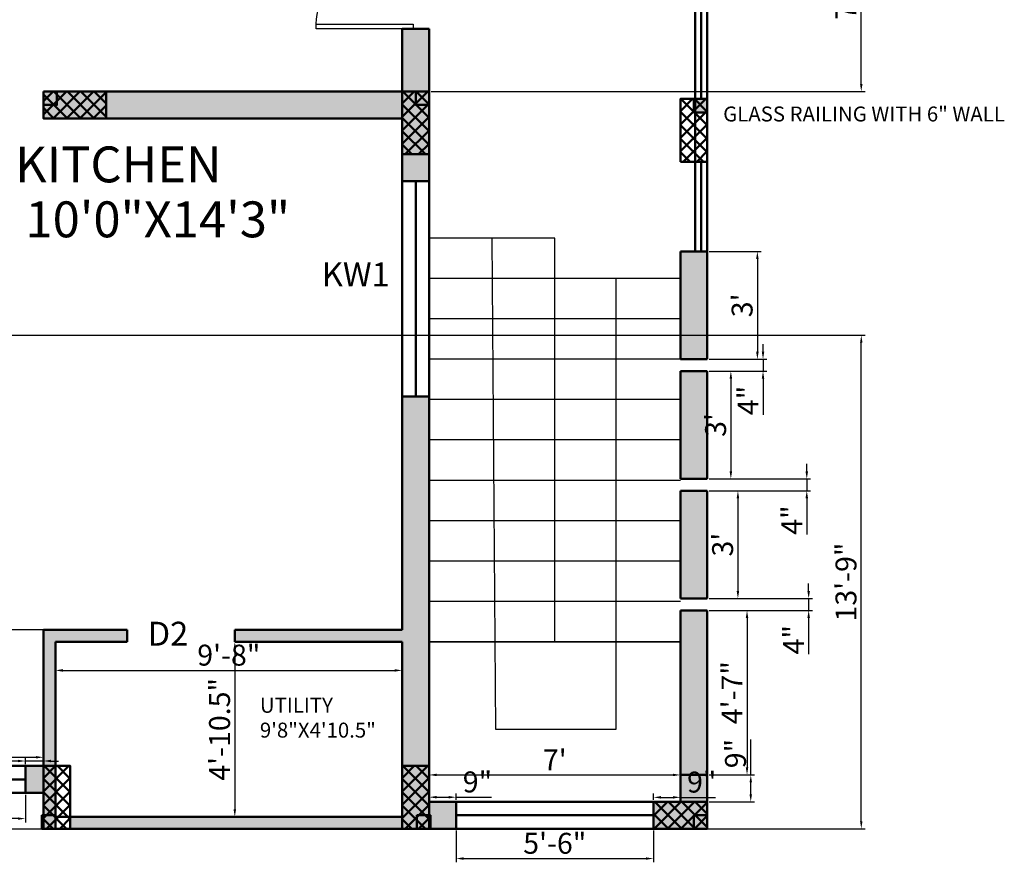
# Model space of a CAD drawing. Units: inches. Extents: x 1749 to 3550, y 1117 to 2383.
# Tile 4 of 15: x 2277 to 2606, y 1199 to 1481. Entities that reach past the tile are written whole.
import ezdxf

# ---------------------------------------------------------------- set-up
doc = ezdxf.new("R2010")
doc.units = ezdxf.units.IN
for name, color, linetype, lineweight in [('A-ANNO-DIMS', 2, 'Continuous', 18), ('A-ANNO-TEXT', 3, 'Continuous', 18), ('A-AREA-IDEN', 7, 'Continuous', 18), ('A-COLS', 10, 'Continuous', 50), ('A-DOOR', 30, 'Continuous', 25), ('A-FLOR-STRS', 53, 'Continuous', 25), ('A-WALL', 7, 'Continuous', 50), ('A-WALL-PATT', 8, 'Continuous', 13)]:
    doc.layers.add(name, color=color, linetype=linetype, lineweight=lineweight)
doc.styles.get("Standard").update_dxf_attribs({"font": 'arial.ttf'})
doc.dimstyles.new('ISO-25', dxfattribs={"dimtxt": 7, "dimasz": 2.5, "dimexe": 1.25, "dimexo": 0.625, "dimtad": 1, "dimdec": 1, "dimlunit": 3, "dimtxsty": 'Standard', "dimcen": 2.5, "dimadec": 0, "dimazin": 0, "dimtfac": 1, "dimtdec": 1, "dimtmove": 0, "dimatfit": 3, "dimfxl": 1, "dimarcsym": 0})

# ---------------------------------------------------------------- blocks, each defined once
blk = doc.blocks.new('*U14')
for p, q in [((0, 0), (0, 6)), ((36, 0), (36, 6))]:
    blk.add_line(p, q)
blk.add_lwpolyline([(0, 0), (0, -36), (1.75, -36), (1.75, 0)], close=True)
blk.add_arc((0, 0), 36, 270, 0)
blk = doc.blocks.new('*D27')
at = {"layer": 'A-ANNO-DIMS', "color": 0, "lineweight": -2, "ltscale": 0.5, "transparency": 16777216}
for p, q in [((2349.73, 1272.74), (2350.35, 1272.74)), ((2349.1, 1270.24), (2349.1, 1216.74)), ((2349.73, 1214.24), (2350.35, 1214.24))]:
    blk.add_line(p, q, dxfattribs=at)
at = {"layer": 'A-ANNO-DIMS', "color": 0, "ltscale": 0.5, "transparency": 16777216}
for points in [[(2348.69, 1270.24), (2349.52, 1270.24), (2349.1, 1272.74)], [(2348.69, 1216.74), (2349.52, 1216.74), (2349.1, 1214.24)]]:
    blk.add_solid(points, dxfattribs=at)
at = {"layer": 'Defpoints', "color": 0, "ltscale": 0.5, "transparency": 16777216}
for p in [(2349.1, 1272.74), (2349.1, 1214.24), (2349.1, 1214.24)]:
    blk.add_point(p, dxfattribs=at)
at = {"layer": 'A-ANNO-DIMS', "color": 0, "ltscale": 0.5, "transparency": 16777216, "insert": (2344.91, 1243.49), "char_height": 7, "attachment_point": 5, "rotation": 90}
blk.add_mtext('4\'-10.5"', dxfattribs=at)
blk = doc.blocks.new('*D28')
at = {"layer": 'A-ANNO-DIMS', "color": 0, "lineweight": -2, "ltscale": 0.5, "transparency": 16777216}
for p, q in [((2289.1, 1272.12), (2289.1, 1261.94)), ((2405.1, 1272.12), (2405.1, 1261.94)), ((2291.6, 1263.19), (2402.6, 1263.19))]:
    blk.add_line(p, q, dxfattribs=at)
at = {"layer": 'A-ANNO-DIMS', "color": 0, "ltscale": 0.5, "transparency": 16777216}
for points in [[(2291.6, 1263.61), (2291.6, 1262.77), (2289.1, 1263.19)], [(2402.6, 1263.61), (2402.6, 1262.77), (2405.1, 1263.19)]]:
    blk.add_solid(points, dxfattribs=at)
at = {"layer": 'Defpoints', "color": 0, "ltscale": 0.5, "transparency": 16777216}
for p in [(2289.1, 1272.74), (2405.1, 1272.74), (2405.1, 1263.19)]:
    blk.add_point(p, dxfattribs=at)
at = {"layer": 'A-ANNO-DIMS', "color": 0, "ltscale": 0.5, "transparency": 16777216, "insert": (2347.1, 1267.39), "char_height": 7, "attachment_point": 5}
blk.add_mtext('9\'-8"', dxfattribs=at)
blk = doc.blocks.new('*D29')
at = {"layer": 'A-ANNO-DIMS', "color": 0, "lineweight": -2, "ltscale": 0.5, "transparency": 16777216}
for p, q in [((2414.1, 1219.87), (2414.1, 1229.49)), ((2416.6, 1228.24), (2495.6, 1228.24)), ((2498.1, 1219.87), (2498.1, 1229.49))]:
    blk.add_line(p, q, dxfattribs=at)
at = {"layer": 'A-ANNO-DIMS', "color": 0, "ltscale": 0.5, "transparency": 16777216}
for points in [[(2416.6, 1228.66), (2416.6, 1227.83), (2414.1, 1228.24)], [(2495.6, 1228.66), (2495.6, 1227.83), (2498.1, 1228.24)]]:
    blk.add_solid(points, dxfattribs=at)
at = {"layer": 'Defpoints', "color": 0, "ltscale": 0.5, "transparency": 16777216}
for p in [(2498.1, 1228.24), (2414.1, 1219.24), (2498.1, 1219.24)]:
    blk.add_point(p, dxfattribs=at)
at = {"layer": 'A-ANNO-DIMS', "color": 0, "ltscale": 0.5, "transparency": 16777216, "insert": (2456.1, 1232.37), "char_height": 7, "attachment_point": 5}
blk.add_mtext("7'", dxfattribs=at)
blk = doc.blocks.new('*D43')
at = {"layer": 'A-ANNO-DIMS', "color": 0, "lineweight": -2, "ltscale": 0.5, "transparency": 16777216}
for p, q in [((2507.73, 1403.24), (2525.11, 1403.24)), ((2523.86, 1400.74), (2523.86, 1369.74)), ((2507.73, 1367.24), (2525.11, 1367.24))]:
    blk.add_line(p, q, dxfattribs=at)
at = {"layer": 'A-ANNO-DIMS', "color": 0, "ltscale": 0.5, "transparency": 16777216}
for points in [[(2523.44, 1400.74), (2524.28, 1400.74), (2523.86, 1403.24)], [(2523.44, 1369.74), (2524.28, 1369.74), (2523.86, 1367.24)]]:
    blk.add_solid(points, dxfattribs=at)
at = {"layer": 'Defpoints', "color": 0, "ltscale": 0.5, "transparency": 16777216}
for p in [(2507.1, 1403.24), (2507.1, 1367.24), (2523.86, 1367.24)]:
    blk.add_point(p, dxfattribs=at)
at = {"layer": 'A-ANNO-DIMS', "color": 0, "ltscale": 0.5, "transparency": 16777216, "insert": (2519.66, 1385.24), "char_height": 7, "attachment_point": 5, "rotation": 90}
blk.add_mtext("3'", dxfattribs=at)
blk = doc.blocks.new('*D44')
at = {"layer": 'A-ANNO-DIMS', "color": 0, "lineweight": -2, "ltscale": 0.5, "transparency": 16777216}
for p, q in [((2525.75, 1369.74), (2525.75, 1372.24)), ((2507.73, 1367.24), (2527, 1367.24)), ((2525.75, 1367.24), (2525.75, 1363.24)), ((2507.73, 1363.24), (2527, 1363.24)), ((2525.75, 1360.74), (2525.75, 1348.67))]:
    blk.add_line(p, q, dxfattribs=at)
at = {"layer": 'A-ANNO-DIMS', "color": 0, "ltscale": 0.5, "transparency": 16777216}
for points in [[(2525.33, 1369.74), (2526.16, 1369.74), (2525.75, 1367.24)], [(2525.33, 1360.74), (2526.16, 1360.74), (2525.75, 1363.24)]]:
    blk.add_solid(points, dxfattribs=at)
at = {"layer": 'Defpoints', "color": 0, "ltscale": 0.5, "transparency": 16777216}
for p in [(2507.1, 1367.24), (2507.1, 1363.24), (2525.75, 1363.24)]:
    blk.add_point(p, dxfattribs=at)
at = {"layer": 'A-ANNO-DIMS', "color": 0, "ltscale": 0.5, "transparency": 16777216, "insert": (2521.62, 1353.45), "char_height": 7, "attachment_point": 5, "rotation": 90}
blk.add_mtext('4"', dxfattribs=at)
blk = doc.blocks.new('*D45')
at = {"layer": 'A-ANNO-DIMS', "color": 0, "lineweight": -2, "ltscale": 0.5, "transparency": 16777216}
for p, q in [((2507.73, 1363.24), (2516.25, 1363.24)), ((2515, 1360.74), (2515, 1329.74)), ((2507.73, 1327.24), (2516.25, 1327.24))]:
    blk.add_line(p, q, dxfattribs=at)
at = {"layer": 'A-ANNO-DIMS', "color": 0, "ltscale": 0.5, "transparency": 16777216}
for points in [[(2514.58, 1360.74), (2515.41, 1360.74), (2515, 1363.24)], [(2514.58, 1329.74), (2515.41, 1329.74), (2515, 1327.24)]]:
    blk.add_solid(points, dxfattribs=at)
at = {"layer": 'Defpoints', "color": 0, "ltscale": 0.5, "transparency": 16777216}
for p in [(2507.1, 1363.24), (2507.1, 1327.24), (2515, 1327.24)]:
    blk.add_point(p, dxfattribs=at)
at = {"layer": 'A-ANNO-DIMS', "color": 0, "ltscale": 0.5, "transparency": 16777216, "insert": (2510.79, 1345.24), "char_height": 7, "attachment_point": 5, "rotation": 90}
blk.add_mtext("3'", dxfattribs=at)
blk = doc.blocks.new('*D46')
at = {"layer": 'A-ANNO-DIMS', "color": 0, "lineweight": -2, "ltscale": 0.5, "transparency": 16777216}
for p, q in [((2540.38, 1329.74), (2540.38, 1332.24)), ((2507.73, 1327.24), (2541.63, 1327.24)), ((2540.38, 1327.24), (2540.38, 1323.24)), ((2507.73, 1323.24), (2541.63, 1323.24)), ((2540.38, 1320.74), (2540.38, 1308.67))]:
    blk.add_line(p, q, dxfattribs=at)
at = {"layer": 'A-ANNO-DIMS', "color": 0, "ltscale": 0.5, "transparency": 16777216}
for points in [[(2539.96, 1329.74), (2540.8, 1329.74), (2540.38, 1327.24)], [(2539.96, 1320.74), (2540.8, 1320.74), (2540.38, 1323.24)]]:
    blk.add_solid(points, dxfattribs=at)
at = {"layer": 'Defpoints', "color": 0, "ltscale": 0.5, "transparency": 16777216}
for p in [(2507.1, 1327.24), (2507.1, 1323.24), (2540.38, 1323.24)]:
    blk.add_point(p, dxfattribs=at)
at = {"layer": 'A-ANNO-DIMS', "color": 0, "ltscale": 0.5, "transparency": 16777216, "insert": (2536.25, 1313.45), "char_height": 7, "attachment_point": 5, "rotation": 90}
blk.add_mtext('4"', dxfattribs=at)
blk = doc.blocks.new('*D47')
at = {"layer": 'A-ANNO-DIMS', "color": 0, "lineweight": -2, "ltscale": 0.5, "transparency": 16777216}
for p, q in [((2507.73, 1323.24), (2518.6, 1323.24)), ((2517.35, 1320.74), (2517.35, 1289.74)), ((2507.73, 1287.24), (2518.6, 1287.24))]:
    blk.add_line(p, q, dxfattribs=at)
at = {"layer": 'A-ANNO-DIMS', "color": 0, "ltscale": 0.5, "transparency": 16777216}
for points in [[(2516.93, 1320.74), (2517.76, 1320.74), (2517.35, 1323.24)], [(2516.93, 1289.74), (2517.76, 1289.74), (2517.35, 1287.24)]]:
    blk.add_solid(points, dxfattribs=at)
at = {"layer": 'Defpoints', "color": 0, "ltscale": 0.5, "transparency": 16777216}
for p in [(2507.1, 1323.24), (2507.1, 1287.24), (2517.35, 1287.24)]:
    blk.add_point(p, dxfattribs=at)
at = {"layer": 'A-ANNO-DIMS', "color": 0, "ltscale": 0.5, "transparency": 16777216, "insert": (2513.14, 1305.24), "char_height": 7, "attachment_point": 5, "rotation": 90}
blk.add_mtext("3'", dxfattribs=at)
blk = doc.blocks.new('*D48')
at = {"layer": 'A-ANNO-DIMS', "color": 0, "lineweight": -2, "ltscale": 0.5, "transparency": 16777216}
for p, q in [((2541.01, 1289.74), (2541.01, 1292.24)), ((2507.73, 1287.24), (2542.26, 1287.24)), ((2541.01, 1287.24), (2541.01, 1283.24)), ((2507.73, 1283.24), (2542.26, 1283.24)), ((2541.01, 1280.74), (2541.01, 1268.67))]:
    blk.add_line(p, q, dxfattribs=at)
at = {"layer": 'A-ANNO-DIMS', "color": 0, "ltscale": 0.5, "transparency": 16777216}
for points in [[(2540.59, 1289.74), (2541.43, 1289.74), (2541.01, 1287.24)], [(2540.59, 1280.74), (2541.43, 1280.74), (2541.01, 1283.24)]]:
    blk.add_solid(points, dxfattribs=at)
at = {"layer": 'Defpoints', "color": 0, "ltscale": 0.5, "transparency": 16777216}
for p in [(2507.1, 1287.24), (2507.1, 1283.24), (2541.01, 1283.24)]:
    blk.add_point(p, dxfattribs=at)
at = {"layer": 'A-ANNO-DIMS', "color": 0, "ltscale": 0.5, "transparency": 16777216, "insert": (2536.88, 1273.45), "char_height": 7, "attachment_point": 5, "rotation": 90}
blk.add_mtext('4"', dxfattribs=at)
blk = doc.blocks.new('*D49')
at = {"layer": 'A-ANNO-DIMS', "color": 0, "lineweight": -2, "ltscale": 0.5, "transparency": 16777216}
for p, q in [((2507.73, 1283.24), (2521.65, 1283.24)), ((2520.4, 1280.74), (2520.4, 1230.74)), ((2507.73, 1228.24), (2521.65, 1228.24))]:
    blk.add_line(p, q, dxfattribs=at)
at = {"layer": 'A-ANNO-DIMS', "color": 0, "ltscale": 0.5, "transparency": 16777216}
for points in [[(2519.98, 1280.74), (2520.81, 1280.74), (2520.4, 1283.24)], [(2519.98, 1230.74), (2520.81, 1230.74), (2520.4, 1228.24)]]:
    blk.add_solid(points, dxfattribs=at)
at = {"layer": 'Defpoints', "color": 0, "ltscale": 0.5, "transparency": 16777216}
for p in [(2507.1, 1283.24), (2507.1, 1228.24), (2520.4, 1228.24)]:
    blk.add_point(p, dxfattribs=at)
at = {"layer": 'A-ANNO-DIMS', "color": 0, "ltscale": 0.5, "transparency": 16777216, "insert": (2516.27, 1255.74), "char_height": 7, "attachment_point": 5, "rotation": 90}
blk.add_mtext('4\'-7"', dxfattribs=at)
blk = doc.blocks.new('*D50')
at = {"layer": 'A-ANNO-DIMS', "color": 0, "lineweight": -2, "ltscale": 0.5, "transparency": 16777216}
for p, q in [((2521.65, 1228.24), (2521.65, 1240.04)), ((2507.73, 1228.24), (2522.9, 1228.24)), ((2521.65, 1221.74), (2521.65, 1225.74)), ((2507.73, 1219.24), (2522.9, 1219.24))]:
    blk.add_line(p, q, dxfattribs=at)
at = {"layer": 'A-ANNO-DIMS', "color": 0, "ltscale": 0.5, "transparency": 16777216}
for points in [[(2521.23, 1225.74), (2522.06, 1225.74), (2521.65, 1228.24)], [(2521.23, 1221.74), (2522.06, 1221.74), (2521.65, 1219.24)]]:
    blk.add_solid(points, dxfattribs=at)
at = {"layer": 'Defpoints', "color": 0, "ltscale": 0.5, "transparency": 16777216}
for p in [(2507.1, 1228.24), (2521.65, 1228.24), (2507.1, 1219.24)]:
    blk.add_point(p, dxfattribs=at)
at = {"layer": 'A-ANNO-DIMS', "color": 0, "ltscale": 0.5, "transparency": 16777216, "insert": (2517.45, 1235.39), "char_height": 7, "attachment_point": 5, "rotation": 90}
blk.add_mtext('9"', dxfattribs=at)
blk = doc.blocks.new('*D51')
at = {"layer": 'A-ANNO-DIMS', "color": 0, "lineweight": -2, "ltscale": 0.5, "transparency": 16777216}
for p, q in [((2414.1, 1219.87), (2414.1, 1222.05)), ((2423.1, 1219.87), (2423.1, 1222.05)), ((2416.6, 1220.8), (2420.6, 1220.8)), ((2423.1, 1220.8), (2434.9, 1220.8))]:
    blk.add_line(p, q, dxfattribs=at)
at = {"layer": 'A-ANNO-DIMS', "color": 0, "ltscale": 0.5, "transparency": 16777216}
for points in [[(2416.6, 1221.21), (2416.6, 1220.38), (2414.1, 1220.8)], [(2420.6, 1221.21), (2420.6, 1220.38), (2423.1, 1220.8)]]:
    blk.add_solid(points, dxfattribs=at)
at = {"layer": 'Defpoints', "color": 0, "ltscale": 0.5, "transparency": 16777216}
for p in [(2414.1, 1219.24), (2423.1, 1220.8), (2423.1, 1219.24)]:
    blk.add_point(p, dxfattribs=at)
at = {"layer": 'A-ANNO-DIMS', "color": 0, "ltscale": 0.5, "transparency": 16777216, "insert": (2430.25, 1225), "char_height": 7, "attachment_point": 5}
blk.add_mtext('9"', dxfattribs=at)
blk = doc.blocks.new('*D52')
at = {"layer": 'A-ANNO-DIMS', "color": 0, "lineweight": -2, "ltscale": 0.5, "transparency": 16777216}
for p, q in [((2423.1, 1209.62), (2423.1, 1199.03)), ((2489.1, 1209.62), (2489.1, 1199.03)), ((2425.6, 1200.28), (2486.6, 1200.28))]:
    blk.add_line(p, q, dxfattribs=at)
at = {"layer": 'A-ANNO-DIMS', "color": 0, "ltscale": 0.5, "transparency": 16777216}
for points in [[(2425.6, 1200.7), (2425.6, 1199.87), (2423.1, 1200.28)], [(2486.6, 1200.7), (2486.6, 1199.87), (2489.1, 1200.28)]]:
    blk.add_solid(points, dxfattribs=at)
at = {"layer": 'Defpoints', "color": 0, "ltscale": 0.5, "transparency": 16777216}
for p in [(2423.1, 1210.24), (2489.1, 1210.24), (2489.1, 1200.28)]:
    blk.add_point(p, dxfattribs=at)
at = {"layer": 'A-ANNO-DIMS', "color": 0, "ltscale": 0.5, "transparency": 16777216, "insert": (2456.1, 1204.48), "char_height": 7, "attachment_point": 5}
blk.add_mtext('5\'-6"', dxfattribs=at)
blk = doc.blocks.new('*D53')
at = {"layer": 'A-ANNO-DIMS', "color": 0, "lineweight": -2, "ltscale": 0.5, "transparency": 16777216}
for p, q in [((2489.1, 1219.87), (2489.1, 1222)), ((2498.1, 1219.87), (2498.1, 1222)), ((2491.6, 1220.75), (2495.6, 1220.75)), ((2498.1, 1220.75), (2509.9, 1220.75))]:
    blk.add_line(p, q, dxfattribs=at)
at = {"layer": 'A-ANNO-DIMS', "color": 0, "ltscale": 0.5, "transparency": 16777216}
for points in [[(2491.6, 1221.17), (2491.6, 1220.33), (2489.1, 1220.75)], [(2495.6, 1221.17), (2495.6, 1220.33), (2498.1, 1220.75)]]:
    blk.add_solid(points, dxfattribs=at)
at = {"layer": 'Defpoints', "color": 0, "ltscale": 0.5, "transparency": 16777216}
for p in [(2489.1, 1219.24), (2498.1, 1220.75), (2498.1, 1219.24)]:
    blk.add_point(p, dxfattribs=at)
at = {"layer": 'A-ANNO-DIMS', "color": 0, "ltscale": 0.5, "transparency": 16777216, "insert": (2505.25, 1224.95), "char_height": 7, "attachment_point": 5}
blk.add_mtext('9"', dxfattribs=at)
blk = doc.blocks.new('*D54')
at = {"layer": 'A-ANNO-DIMS', "color": 0, "lineweight": -2, "ltscale": 0.5, "transparency": 16777216}
for p, q in [((2276.6, 1232.9), (2264.77, 1232.9)), ((2279.1, 1231.87), (2279.1, 1234.15)), ((2285.1, 1232.9), (2279.1, 1232.9)), ((2285.1, 1231.87), (2285.1, 1234.15)), ((2287.6, 1232.9), (2290.1, 1232.9))]:
    blk.add_line(p, q, dxfattribs=at)
at = {"layer": 'A-ANNO-DIMS', "color": 0, "ltscale": 0.5, "transparency": 16777216}
for points in [[(2276.6, 1233.32), (2276.6, 1232.49), (2279.1, 1232.9)], [(2287.6, 1233.32), (2287.6, 1232.49), (2285.1, 1232.9)]]:
    blk.add_solid(points, dxfattribs=at)
at = {"layer": 'Defpoints', "color": 0, "ltscale": 0.5, "transparency": 16777216}
for p in [(2279.1, 1232.9), (2279.1, 1231.24), (2285.1, 1231.24)]:
    blk.add_point(p, dxfattribs=at)
at = {"layer": 'A-ANNO-DIMS', "color": 0, "ltscale": 0.5, "transparency": 16777216, "insert": (2269.44, 1237.1), "char_height": 7, "attachment_point": 5}
blk.add_mtext('6"', dxfattribs=at)
blk = doc.blocks.new('*D55')
at = {"layer": 'A-ANNO-DIMS', "color": 0, "lineweight": -2, "ltscale": 0.5, "transparency": 16777216}
for p, q in [((2255.1, 1221.62), (2255.1, 1212.39)), ((2279.1, 1221.62), (2279.1, 1212.39)), ((2276.6, 1213.64), (2257.6, 1213.64))]:
    blk.add_line(p, q, dxfattribs=at)
at = {"layer": 'A-ANNO-DIMS', "color": 0, "ltscale": 0.5, "transparency": 16777216}
for points in [[(2257.6, 1214.06), (2257.6, 1213.23), (2255.1, 1213.64)], [(2276.6, 1214.06), (2276.6, 1213.23), (2279.1, 1213.64)]]:
    blk.add_solid(points, dxfattribs=at)
at = {"layer": 'Defpoints', "color": 0, "ltscale": 0.5, "transparency": 16777216}
for p in [(2255.1, 1222.24), (2279.1, 1222.24), (2255.1, 1213.64)]:
    blk.add_point(p, dxfattribs=at)
at = {"layer": 'A-ANNO-DIMS', "color": 0, "ltscale": 0.5, "transparency": 16777216, "insert": (2267.1, 1217.78), "char_height": 7, "attachment_point": 5}
blk.add_mtext("2'", dxfattribs=at)
blk = doc.blocks.new('*D150')
at = {"layer": 'A-ANNO-DIMS', "color": 0, "lineweight": -2, "ltscale": 0.5, "transparency": 16777216}
for p, q in [((2103.6, 1231.87), (2103.6, 1235.4)), ((2285.1, 1231.87), (2285.1, 1235.4)), ((2106.1, 1234.15), (2282.6, 1234.15))]:
    blk.add_line(p, q, dxfattribs=at)
at = {"layer": 'A-ANNO-DIMS', "color": 0, "ltscale": 0.5, "transparency": 16777216}
for points in [[(2106.1, 1234.57), (2106.1, 1233.74), (2103.6, 1234.15)], [(2282.6, 1234.57), (2282.6, 1233.74), (2285.1, 1234.15)]]:
    blk.add_solid(points, dxfattribs=at)
at = {"layer": 'Defpoints', "color": 0, "ltscale": 0.5, "transparency": 16777216}
for p in [(2285.1, 1234.15), (2103.6, 1231.24), (2285.1, 1231.24)]:
    blk.add_point(p, dxfattribs=at)
at = {"layer": 'A-ANNO-DIMS', "color": 0, "ltscale": 0.5, "transparency": 16777216, "insert": (2194.35, 1238.35), "char_height": 7, "attachment_point": 5}
blk.add_mtext('15\'-1.5"', dxfattribs=at)
blk = doc.blocks.new('*D174')
at = {"layer": 'A-ANNO-DIMS', "color": 0, "lineweight": -2, "ltscale": 0.5, "transparency": 16777216}
for p, q in [((2519.23, 1542.24), (2559.85, 1542.24)), ((2558.6, 1459.24), (2558.6, 1539.74)), ((2414.73, 1456.74), (2559.85, 1456.74))]:
    blk.add_line(p, q, dxfattribs=at)
at = {"layer": 'A-ANNO-DIMS', "color": 0, "ltscale": 0.5, "transparency": 16777216}
for points in [[(2558.19, 1539.74), (2559.02, 1539.74), (2558.6, 1542.24)], [(2558.19, 1459.24), (2559.02, 1459.24), (2558.6, 1456.74)]]:
    blk.add_solid(points, dxfattribs=at)
at = {"layer": 'Defpoints', "color": 0, "ltscale": 0.5, "transparency": 16777216}
for p in [(2518.6, 1542.24), (2558.6, 1542.24), (2414.1, 1456.74)]:
    blk.add_point(p, dxfattribs=at)
at = {"layer": 'A-ANNO-DIMS', "color": 0, "ltscale": 0.5, "transparency": 16777216, "insert": (2554.36, 1499.49), "char_height": 7, "attachment_point": 5, "rotation": 90}
blk.add_mtext('7\'-1 1/2"', dxfattribs=at)
blk = doc.blocks.new('*D179')
at = {"layer": 'A-ANNO-DIMS', "color": 0, "lineweight": -2, "ltscale": 0.5, "transparency": 16777216}
for p, q in [((2113.73, 1375.24), (2559.85, 1375.24)), ((2558.6, 1212.74), (2558.6, 1372.74)), ((2104.23, 1210.24), (2559.85, 1210.24))]:
    blk.add_line(p, q, dxfattribs=at)
at = {"layer": 'A-ANNO-DIMS', "color": 0, "ltscale": 0.5, "transparency": 16777216}
for points in [[(2558.19, 1372.74), (2559.02, 1372.74), (2558.6, 1375.24)], [(2558.19, 1212.74), (2559.02, 1212.74), (2558.6, 1210.24)]]:
    blk.add_solid(points, dxfattribs=at)
at = {"layer": 'Defpoints', "color": 0, "ltscale": 0.5, "transparency": 16777216}
for p in [(2113.1, 1375.24), (2558.6, 1375.24), (2103.6, 1210.24)]:
    blk.add_point(p, dxfattribs=at)
at = {"layer": 'A-ANNO-DIMS', "color": 0, "ltscale": 0.5, "transparency": 16777216, "insert": (2554.4, 1292.74), "char_height": 7, "attachment_point": 5, "rotation": 90}
blk.add_mtext('13\'-9"', dxfattribs=at)

msp = doc.modelspace()

# ---------------------------------------------------------------- hatches: boundary and pattern name
at = {"layer": 'A-COLS', "ltscale": 10}
h = msp.add_hatch(color=256, dxfattribs=at)
h.dxf.hatch_style = 1
h.paths.add_polyline_path([(2285.1, 1456.74), (2285.1, 1452.24), (2289.6, 1452.24), (2289.6, 1456.74)])
h = msp.add_hatch(dxfattribs=at)
h.set_pattern_fill('ANSI37', color=256)
h.set_pattern_definition([(45, (633.86, 89.6368), (-2.245064, 2.245064), []), (135, (633.86, 89.6368), (-2.245064, -2.245064), [])])
h.paths.add_polyline_path([(2306.1, 1447.74), (2306.1, 1456.74), (2285.1, 1456.74), (2285.1, 1447.74)])
h = msp.add_hatch(dxfattribs=at)
h.set_pattern_fill('ANSI37', color=256, angle=90)
h.set_pattern_definition([(135, (3772.2103, -215.5015), (-2.245064, -2.245064), []), (225, (3772.2103, -215.5015), (2.245064, -2.245064), [])])
h.paths.add_polyline_path([(2414.1, 1456.74), (2405.1, 1456.74), (2405.1, 1435.74), (2414.1, 1435.74)])
h = msp.add_hatch(color=256, dxfattribs=at)
h.dxf.hatch_style = 1
h.paths.add_polyline_path([(2409.6, 1456.74), (2409.6, 1452.24), (2414.1, 1452.24), (2414.1, 1456.74)])
h = msp.add_hatch(dxfattribs=at)
h.set_pattern_fill('ANSI37', color=256, angle=90)
h.set_pattern_definition([(135, (3865.2103, -218.0015), (-2.245064, -2.245064), []), (225, (3865.2103, -218.0015), (2.245064, -2.245064), [])])
h.paths.add_polyline_path([(2507.1, 1454.24), (2498.1, 1454.24), (2498.1, 1433.24), (2507.1, 1433.24)])
h = msp.add_hatch(color=256, dxfattribs=at)
h.dxf.hatch_style = 1
h.paths.add_polyline_path([(2502.6, 1454.24), (2502.6, 1449.74), (2507.1, 1449.74), (2507.1, 1454.24)])
h = msp.add_hatch(dxfattribs=at)
h.set_pattern_fill('ANSI37', color=256, angle=90)
h.set_pattern_definition([(135, (3652.2103, -441.0015), (-2.245064, -2.245064), []), (225, (3652.2103, -441.0015), (2.245064, -2.245064), [])])
h.paths.add_polyline_path([(2294.1, 1231.24), (2285.1, 1231.24), (2285.1, 1210.24), (2294.1, 1210.24)])
h = msp.add_hatch(dxfattribs=at)
h.set_pattern_fill('ANSI37', color=256, angle=90)
h.set_pattern_definition([(135, (3772.2103, -441.0015), (-2.245064, -2.245064), []), (225, (3772.2103, -441.0015), (2.245064, -2.245064), [])])
h.paths.add_polyline_path([(2414.1, 1231.24), (2405.1, 1231.24), (2405.1, 1210.24), (2414.1, 1210.24)])
h = msp.add_hatch(dxfattribs=at)
h.set_pattern_fill('ANSI37', color=256)
h.set_pattern_definition([(45, (834.86, -147.8632), (-2.245064, 2.245064), []), (135, (834.86, -147.8632), (-2.245064, -2.245064), [])])
h.paths.add_polyline_path([(2507.1, 1210.24), (2507.1, 1219.24), (2489.1, 1219.24), (2489.1, 1210.24)])
h = msp.add_hatch(color=256, dxfattribs=at)
h.dxf.hatch_style = 1
h.paths.add_polyline_path([(2284.6, 1214.74), (2284.6, 1210.24), (2289.1, 1210.24), (2289.1, 1214.74)])
h = msp.add_hatch(color=256, dxfattribs=at)
h.dxf.hatch_style = 1
h.paths.add_polyline_path([(2410, 1214.74), (2410, 1210.24), (2414.5, 1210.24), (2414.5, 1214.74)])
h = msp.add_hatch(color=256, dxfattribs=at)
h.dxf.hatch_style = 1
h.paths.add_polyline_path([(2502.6, 1214.74), (2502.6, 1210.24), (2507.1, 1210.24), (2507.1, 1214.74)])
at = {"layer": 'A-WALL-PATT', "ltscale": 10}
h = msp.add_hatch(color=256, dxfattribs=at)
h.dxf.hatch_style = 1
h.paths.add_polyline_path([(2405.1, 1447.74), (2405.1, 1426.74), (2414.1, 1426.74), (2414.1, 1477.74), (2405.1, 1477.74), (2405.1, 1456.74), (2285.1, 1456.74), (2285.1, 1447.74)])
h = msp.add_hatch(color=256, dxfattribs=at)
h.dxf.hatch_style = 1
h.paths.add_polyline_path([(2498.1, 1367.24), (2507.1, 1367.24), (2507.1, 1403.24), (2498.1, 1403.24)])
h.paths.add_polyline_path([(2507.1, 1363.24), (2498.1, 1363.24), (2498.1, 1327.24), (2507.1, 1327.24)])
h.paths.add_polyline_path([(2507.1, 1323.24), (2498.1, 1323.24), (2498.1, 1287.24), (2507.1, 1287.24)])
h = msp.add_hatch(color=256, dxfattribs=at)
h.dxf.hatch_style = 1
h.paths.add_polyline_path([(2414.1, 1354.74), (2405.1, 1354.74), (2405.1, 1276.74), (2349.1, 1276.74), (2349.1, 1272.74), (2405.1, 1272.74), (2405.1, 1214.24), (2405.1, 1210.24), (2423.1, 1210.24), (2423.1, 1219.24), (2414.1, 1219.24)])
h = msp.add_hatch(color=256, dxfattribs=at)
h.dxf.hatch_style = 1
h.paths.add_polyline_path([(2498.1, 1228.24), (2507.1, 1228.24), (2507.1, 1283.24), (2498.1, 1283.24)])
h = msp.add_hatch(color=256, dxfattribs=at)
h.dxf.hatch_style = 1
h.paths.add_polyline_path([(2285.1, 1276.74), (2285.1, 1231.24), (2279.1, 1231.24), (2279.1, 1222.24), (2285.1, 1222.24), (2285.1, 1210.24), (2289.1, 1210.24), (2289.1, 1214.24), (2289.1, 1272.74), (2313.1, 1272.74), (2313.1, 1276.74)])
h = msp.add_hatch(color=256, dxfattribs=at)
h.dxf.hatch_style = 1
h.paths.add_polyline_path([(2507.1, 1210.24), (2507.1, 1228.24), (2498.1, 1228.24), (2498.1, 1219.24), (2489.1, 1219.24), (2489.1, 1210.24)])
h = msp.add_hatch(color=256, dxfattribs=at)
h.dxf.hatch_style = 1
h.paths.add_polyline_path([(2405.1, 1214.24), (2294.1, 1214.24), (2294.1, 1210.24), (2405.1, 1210.24)])

# ---------------------------------------------------------------- linework, layer by layer
at = {"layer": 'A-COLS', "ltscale": 10}
for points in [[(2285.1, 1456.74), (2289.6, 1456.74), (2289.6, 1452.24), (2285.1, 1452.24)], [(2285.1, 1456.74), (2306.1, 1456.74), (2306.1, 1447.74), (2285.1, 1447.74)], [(2405.1, 1435.74), (2405.1, 1456.74), (2414.1, 1456.74), (2414.1, 1435.74)], [(2409.6, 1456.74), (2414.1, 1456.74), (2414.1, 1452.24), (2409.6, 1452.24)], [(2498.1, 1433.24), (2498.1, 1454.24), (2507.1, 1454.24), (2507.1, 1433.24)], [(2502.6, 1454.24), (2507.1, 1454.24), (2507.1, 1449.74), (2502.6, 1449.74)], [(2285.1, 1210.24), (2285.1, 1231.24), (2294.1, 1231.24), (2294.1, 1210.24)], [(2405.1, 1210.24), (2405.1, 1231.24), (2414.1, 1231.24), (2414.1, 1210.24)], [(2489.1, 1219.24), (2507.1, 1219.24), (2507.1, 1210.24), (2489.1, 1210.24)], [(2284.6, 1214.74), (2289.1, 1214.74), (2289.1, 1210.24), (2284.6, 1210.24)], [(2410, 1214.74), (2414.5, 1214.74), (2414.5, 1210.24), (2410, 1210.24)], [(2502.6, 1214.74), (2507.1, 1214.74), (2507.1, 1210.24), (2502.6, 1210.24)]]:
    msp.add_lwpolyline(points, close=True, dxfattribs=at)
at = {"layer": 'A-FLOR-STRS', "ltscale": 0.5}
for p, q in [((2456.13, 1407.74), (2414.1, 1407.74)), ((2436.4, 1243.46), (2435.12, 1407.74)), ((2456.13, 1394.24), (2456.13, 1407.74)), ((2498.1, 1403.24), (2498.16, 1394.24)), ((2498.16, 1394.24), (2414.1, 1394.24)), ((2456.13, 1272.74), (2456.13, 1394.24)), ((2476.48, 1394.24), (2476.48, 1243.46)), ((2498.16, 1380.74), (2414.1, 1380.74)), ((2498.16, 1367.24), (2414.1, 1367.24)), ((2498.16, 1353.74), (2414.1, 1353.74)), ((2498.16, 1340.24), (2414.1, 1340.24)), ((2498.16, 1326.74), (2414.1, 1326.74)), ((2498.16, 1313.24), (2414.1, 1313.24)), ((2498.16, 1299.74), (2414.1, 1299.74)), ((2498.16, 1286.24), (2414.1, 1286.24)), ((2285.1, 1276.74), (2139.6, 1276.74)), ((2414.1, 1272.74), (2498.1, 1272.74)), ((2498.16, 1272.74), (2414.1, 1272.74)), ((2476.48, 1243.46), (2436.4, 1243.46))]:
    msp.add_line(p, q, dxfattribs=at)
at = {"layer": 'A-WALL', "ltscale": 0.2}
for p, q in [((2503.1, 1403.24), (2503.1, 1542.24)), ((2505.1, 1454.24), (2505.1, 1542.24)), ((2507.1, 1542.24), (2507.1, 1367.24)), ((2405.1, 1477.74), (2405.1, 1456.74)), ((2405.1, 1477.74), (2414.1, 1477.74)), ((2414.1, 1477.74), (2414.1, 1219.24)), ((2285.1, 1456.74), (2405.1, 1456.74)), ((2285.1, 1447.74), (2285.1, 1456.74)), ((2507.1, 1454.24), (2503.1, 1454.24)), ((2285.1, 1447.74), (2405.1, 1447.74)), ((2405.1, 1447.74), (2405.1, 1276.74)), ((2507.1, 1433.24), (2503.1, 1433.24)), ((2505.1, 1433.24), (2505.1, 1403.24)), ((2405.1, 1426.74), (2414.1, 1426.74)), ((2409.6, 1354.74), (2409.6, 1426.74)), ((2498.1, 1403.24), (2507.1, 1403.24)), ((2498.1, 1403.24), (2498.1, 1367.24)), ((2498.1, 1367.24), (2507.1, 1367.24)), ((2498.1, 1363.24), (2507.1, 1363.24)), ((2498.1, 1363.24), (2498.1, 1327.24)), ((2507.1, 1363.24), (2507.1, 1327.24)), ((2405.1, 1354.74), (2414.1, 1354.74)), ((2498.1, 1327.24), (2507.1, 1327.24)), ((2498.1, 1323.24), (2507.1, 1323.24)), ((2498.1, 1323.24), (2498.1, 1287.24)), ((2507.1, 1323.24), (2507.1, 1287.24)), ((2498.1, 1287.24), (2507.1, 1287.24)), ((2498.1, 1283.24), (2507.1, 1283.24)), ((2498.1, 1283.24), (2498.1, 1219.24)), ((2507.1, 1283.24), (2507.1, 1210.24)), ((2285.1, 1276.74), (2285.1, 1231.24)), ((2285.1, 1276.74), (2313.1, 1276.74)), ((2313.1, 1272.74), (2313.1, 1276.74)), ((2349.1, 1272.74), (2349.1, 1276.74)), ((2349.1, 1276.74), (2405.1, 1276.74)), ((2289.1, 1272.74), (2289.1, 1214.24)), ((2289.1, 1272.74), (2313.1, 1272.74)), ((2349.1, 1272.74), (2405.1, 1272.74)), ((2405.1, 1272.74), (2405.1, 1214.24)), ((2103.6, 1231.24), (2285.1, 1231.24)), ((2279.1, 1231.24), (2279.1, 1222.24)), ((2255.1, 1226.74), (2279.1, 1226.74)), ((2103.6, 1222.24), (2285.1, 1222.24)), ((2285.1, 1222.24), (2285.1, 1210.24)), ((2414.1, 1219.24), (2498.1, 1219.24)), ((2423.1, 1219.24), (2423.1, 1210.24)), ((2489.1, 1219.24), (2489.1, 1210.24)), ((2289.1, 1214.24), (2405.1, 1214.24)), ((2423.1, 1214.74), (2489.1, 1214.74)), ((2285.1, 1210.24), (2496.1, 1210.24)), ((2489.1, 1210.24), (2507.1, 1210.24))]:
    msp.add_line(p, q, dxfattribs=at)
at = {"layer": 'A-WALL', "ltscale": 10}
for p, q in [((2498.1, 1228.24), (2507.1, 1228.24)), ((2289.1, 1214.24), (2289.1, 1210.24)), ((2405.1, 1214.24), (2405.1, 1210.24))]:
    msp.add_line(p, q, dxfattribs=at)

# ---------------------------------------------------------------- block references
at = {"layer": 'A-DOOR', "xscale": -0.9, "yscale": 0.9, "zscale": 0.9, "rotation": 270}
msp.add_blockref('*U14', (2408.7, 1477.74), dxfattribs=at)

# ---------------------------------------------------------------- texts
at = {"layer": 'A-ANNO-TEXT', "ltscale": 0.5}
for s, p in [('KW1', (2378.21, 1391.6)), ('D2', (2319.98, 1271.46))]:
    msp.add_text(s, height=8, dxfattribs=at).set_placement(p)
at = {"layer": 'A-AREA-IDEN', "ltscale": 0.5}
for s, height, p in [('GLASS RAILING WITH 6" WALL', 5, (2512.42, 1446.73)), ('10\'0"X14\'3"', 12, (2279.1, 1408)), ('UTILITY', 5, (2357.5, 1249.03)), ('9\'8"X4\'10.5"', 5, (2357.5, 1240.73))]:
    msp.add_text(s, height=height, dxfattribs=at).set_placement(p)
msp.add_text('KITCHEN', height=12, rotation=0.0333, dxfattribs=at).set_placement((2275.64, 1426.35))

# ---------------------------------------------------------------- dimensions: what is measured, and where the dimension line sits
at = {"layer": 'A-ANNO-DIMS', "ltscale": 0.5}
for base, p1, p2, override, picture, middle in [((2558.6, 1542.24), (2414.1, 1456.74), (2518.6, 1542.24), {"dimdec": 1, "dimlfac": 1, "dimrnd": 0, "dimzin": 1, "dimdsep": 46, "dimlunit": 4, "dimfrac": 2}, '*D174', (2554.36, 1499.49)), ((2523.86, 1367.24), (2507.1, 1403.24), (2507.1, 1367.24), {"dimclrd": 0, "dimclre": 0, "dimclrt": 0}, '*D43', (2519.66, 1385.24)), ((2558.6, 1375.24), (2103.6, 1210.24), (2113.1, 1375.24), {"dimdec": 1, "dimlfac": 1, "dimrnd": 0, "dimzin": 1, "dimdsep": 46, "dimlunit": 4, "dimfrac": 2}, '*D179', (2554.4, 1292.74)), ((2525.75, 1363.24), (2507.1, 1367.24), (2507.1, 1363.24), {"dimclrd": 0, "dimclre": 0, "dimclrt": 0}, '*D44', (2521.62, 1353.45)), ((2515, 1327.24), (2507.1, 1363.24), (2507.1, 1327.24), {"dimclrd": 0, "dimclre": 0, "dimclrt": 0}, '*D45', (2510.79, 1345.24)), ((2540.38, 1323.24), (2507.1, 1327.24), (2507.1, 1323.24), {"dimclrd": 0, "dimclre": 0, "dimclrt": 0}, '*D46', (2536.25, 1313.45)), ((2517.35, 1287.24), (2507.1, 1323.24), (2507.1, 1287.24), {"dimclrd": 0, "dimclre": 0, "dimclrt": 0}, '*D47', (2513.14, 1305.24)), ((2541.01, 1283.24), (2507.1, 1287.24), (2507.1, 1283.24), {"dimclrd": 0, "dimclre": 0, "dimclrt": 0}, '*D48', (2536.88, 1273.45)), ((2520.4, 1228.24), (2507.1, 1283.24), (2507.1, 1228.24), {"dimclrd": 0, "dimclre": 0, "dimclrt": 0}, '*D49', (2516.27, 1255.74)), ((2349.1, 1214.24), (2349.1, 1272.74), (2349.1, 1214.24), {"dimclrd": 0, "dimclre": 0, "dimclrt": 0}, '*D27', (2344.91, 1243.49)), ((2521.65, 1228.24), (2507.1, 1219.24), (2507.1, 1228.24), {"dimclrd": 0, "dimclre": 0, "dimclrt": 0}, '*D50', (2517.45, 1235.39))]:
    dim = msp.add_linear_dim(base=base, p1=p1, p2=p2, angle=90, dimstyle='ISO-25', override=override, dxfattribs=at)
    dim.commit()
    dim.dimension.update_dxf_attribs({"geometry": picture, "text_midpoint": middle})
for base, p1, p2, picture, middle in [((2405.1, 1263.19), (2289.1, 1272.74), (2405.1, 1272.74), '*D28', (2347.1, 1267.39)), ((2285.1, 1234.15), (2103.6, 1231.24), (2285.1, 1231.24), '*D150', (2194.35, 1238.35)), ((2279.1, 1232.9), (2285.1, 1231.24), (2279.1, 1231.24), '*D54', (2269.44, 1237.1)), ((2498.1, 1228.24), (2414.1, 1219.24), (2498.1, 1219.24), '*D29', (2456.1, 1232.37)), ((2423.1, 1220.8), (2414.1, 1219.24), (2423.1, 1219.24), '*D51', (2430.25, 1225)), ((2498.1, 1220.75), (2489.1, 1219.24), (2498.1, 1219.24), '*D53', (2505.25, 1224.95)), ((2255.1, 1213.64), (2279.1, 1222.24), (2255.1, 1222.24), '*D55', (2267.1, 1217.78)), ((2489.1, 1200.28), (2423.1, 1210.24), (2489.1, 1210.24), '*D52', (2456.1, 1204.48))]:
    dim = msp.add_linear_dim(base=base, p1=p1, p2=p2, dimstyle='ISO-25', override={"dimclrd": 0, "dimclre": 0, "dimclrt": 0}, dxfattribs=at)
    dim.commit()
    dim.dimension.update_dxf_attribs({"geometry": picture, "text_midpoint": middle})

doc.saveas('drawing.dxf')
